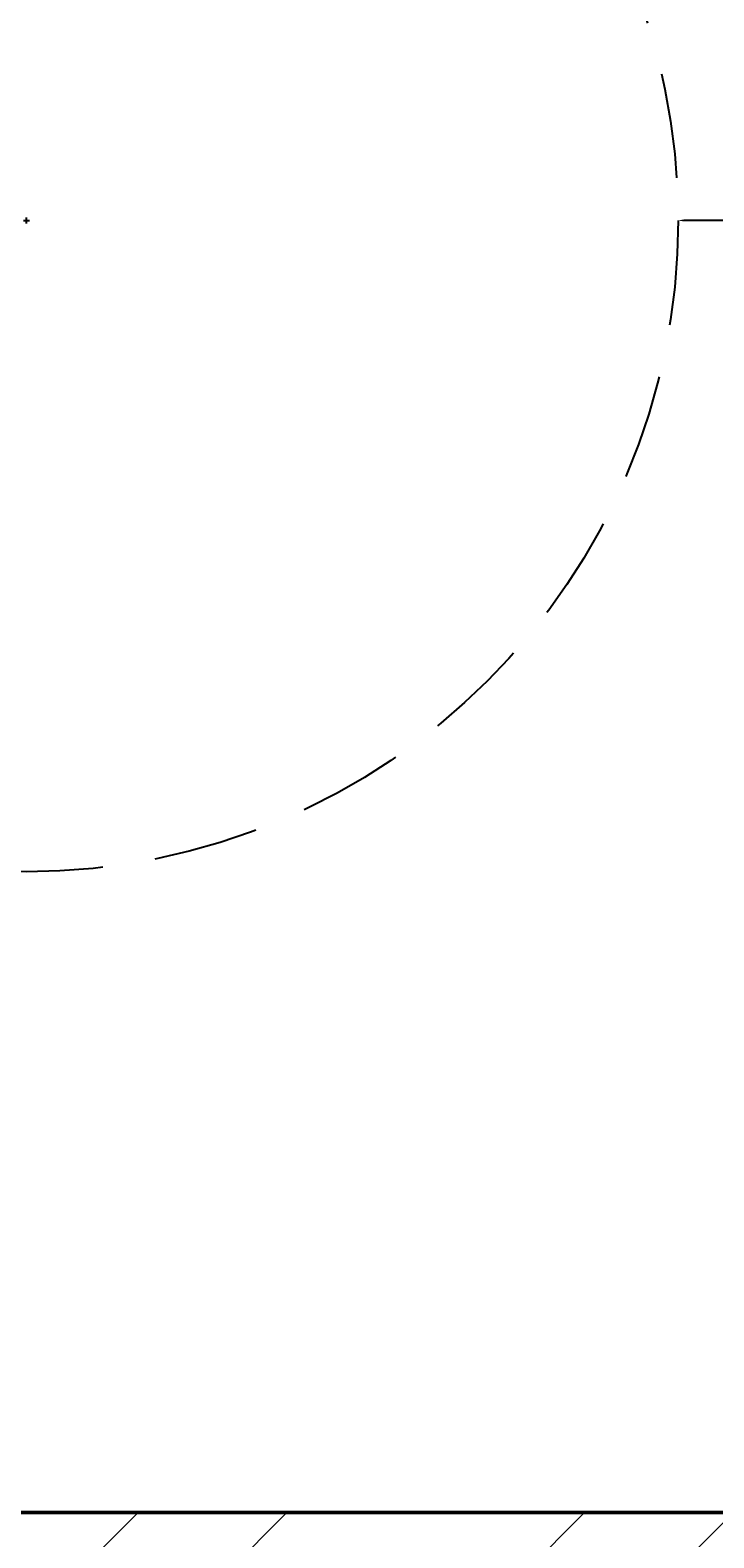
# Model space of a CAD drawing. Units: inches. Extents: x 2812 to 3051, y 1398 to 1659.
# Tile 60 of 65: x 2984 to 3005, y 1559 to 1605. Entities that reach past the tile are written whole.
import ezdxf

# ---------------------------------------------------------------- set-up
doc = ezdxf.new("R2010")
doc.units = ezdxf.units.IN
doc.linetypes.add('HIDDEN2', pattern=[4.7625, 3.175, -1.5875])
for name, color, linetype, lineweight in [('A-ANNO-DIMS', 2, 'Continuous', 18), ('S-CONC', 7, 'Continuous', 50), ('S-CONC-HIDN', 8, 'HIDDEN2', 25), ('S-CONC-PATT', 8, 'Continuous', 18)]:
    doc.layers.add(name, color=color, linetype=linetype, lineweight=lineweight)
doc.styles.get("Standard").update_dxf_attribs({"font": 'arial.ttf'})
doc.dimstyles.get("Standard").update_dxf_attribs({"dimtxt": 0.18, "dimasz": 0.18, "dimexe": 0.18, "dimexo": 0.0625, "dimgap": 0.09, "dimtad": 0, "dimtih": 1, "dimtoh": 1, "dimdec": 4, "dimzin": 0, "dimdsep": 46, "dimtxsty": 'Standard', "dimcen": 0.09, "dimadec": 0, "dimazin": 0, "dimtfac": 1, "dimtdec": 4, "dimtofl": 0, "dimtmove": 0, "dimatfit": 3, "dimfxl": 1, "dimtolj": 1, "dimtzin": 0, "dimarcsym": 0})

# ---------------------------------------------------------------- blocks, each defined once
blk = doc.blocks.new('*D83')
at = {"layer": 'A-ANNO-DIMS', "color": 0, "lineweight": -2, "transparency": 16777216}
for p, q in [((2984.226, 1598.82), (2984.406, 1598.82)), ((2984.316, 1598.73), (2984.316, 1598.91)), ((3015.77, 1598.82), (3004.154, 1598.82))]:
    blk.add_line(p, q, dxfattribs=at)
at = {"layer": 'A-ANNO-DIMS', "color": 0, "transparency": 16777216}
blk.add_solid([(3004.154, 1598.85), (3004.154, 1598.79), (3003.974, 1598.82)], dxfattribs=at)
at = {"layer": 'Defpoints', "color": 0, "transparency": 16777216}
for p in [(2964.657, 1598.82), (3003.974, 1598.82)]:
    blk.add_point(p, dxfattribs=at)
at = {"layer": 'A-ANNO-DIMS', "color": 0, "transparency": 16777216, "insert": (3016.26, 1598.82), "char_height": 0.18, "attachment_point": 5}
blk.add_mtext('\\A1;∅39.32', dxfattribs=at)

msp = doc.modelspace()

# ---------------------------------------------------------------- hatches: boundary and pattern name
at = {"layer": 'S-CONC-PATT'}
h = msp.add_hatch(dxfattribs=at)
h.set_pattern_fill('ANSI32', color=256)
h.paths.add_polyline_path([(3027.3849, 1646.82), (2835.3849, 1646.82), (2835.3849, 1603.2296), (2844.3849, 1603.2296), (2844.3849, 1637.82), (3018.3849, 1637.82), (3018.3849, 1602.5441), (3027.3849, 1602.5441)])
h.paths.add_polyline_path([(2844.3849, 1594.2296), (2835.3849, 1594.2296), (2835.3849, 1550.82), (3027.3849, 1550.82), (3027.3849, 1593.5441), (3018.3849, 1593.5441), (3018.3849, 1559.82), (2844.3849, 1559.82)])
h.paths.add_polyline_path([(2844.3849, 1482.0354), (2835.3849, 1482.0354), (2835.3849, 1463.4959), (2844.3849, 1463.4959)])
h.paths.add_polyline_path([(2844.3849, 1461.4959), (2835.3849, 1461.4959), (2835.3849, 1416.0354), (2844.3849, 1416.0354)])
h.paths.add_polyline_path([(3027.3849, 1482.0354), (3018.3849, 1482.0354), (3018.3849, 1463.2854), (3027.3849, 1463.2854)])
h.paths.add_polyline_path([(3027.3849, 1461.2854), (3018.3849, 1461.2854), (3018.3849, 1416.0354), (3027.3849, 1416.0354)])
h.paths.add_polyline_path([(2961.3849, 1448.4738), (2952.3849, 1448.4738), (2952.3849, 1416.0354), (2961.3849, 1416.0354)])
h.paths.add_polyline_path([(2961.3849, 1462.3026), (2952.3849, 1462.3026), (2952.3849, 1450.4738), (2961.3849, 1450.4738)])
h.paths.add_polyline_path([(2961.3849, 1472.0354), (2952.3849, 1472.0354), (2952.3849, 1462.3026), (2961.3849, 1462.3026)])

# ---------------------------------------------------------------- linework, layer by layer
at = {"layer": 'S-CONC'}
msp.add_line((2844.3849, 1559.82), (3018.3849, 1559.82), dxfattribs=at)
at = {"layer": 'S-CONC-HIDN'}
msp.add_circle((2984.3156, 1598.82), 19.6588, dxfattribs=at)

# ---------------------------------------------------------------- dimensions: what is measured, and where the dimension line sits
at = {"layer": 'A-ANNO-DIMS'}
dim = msp.add_diameter_dim_2p(p1=(2964.6569, 1598.8199), p2=(3003.9744, 1598.82), dimstyle='Standard', override={"dimdec": 2, "dimlfac": 1, "dimrnd": 0, "dimzin": 0, "dimdsep": 46, "dimlunit": 2}, dxfattribs=at)
dim.commit()
dim.dimension.update_dxf_attribs({"geometry": '*D83', "text_midpoint": (3015.7697, 1598.82), "dimtype": 163})

doc.saveas('drawing.dxf')
